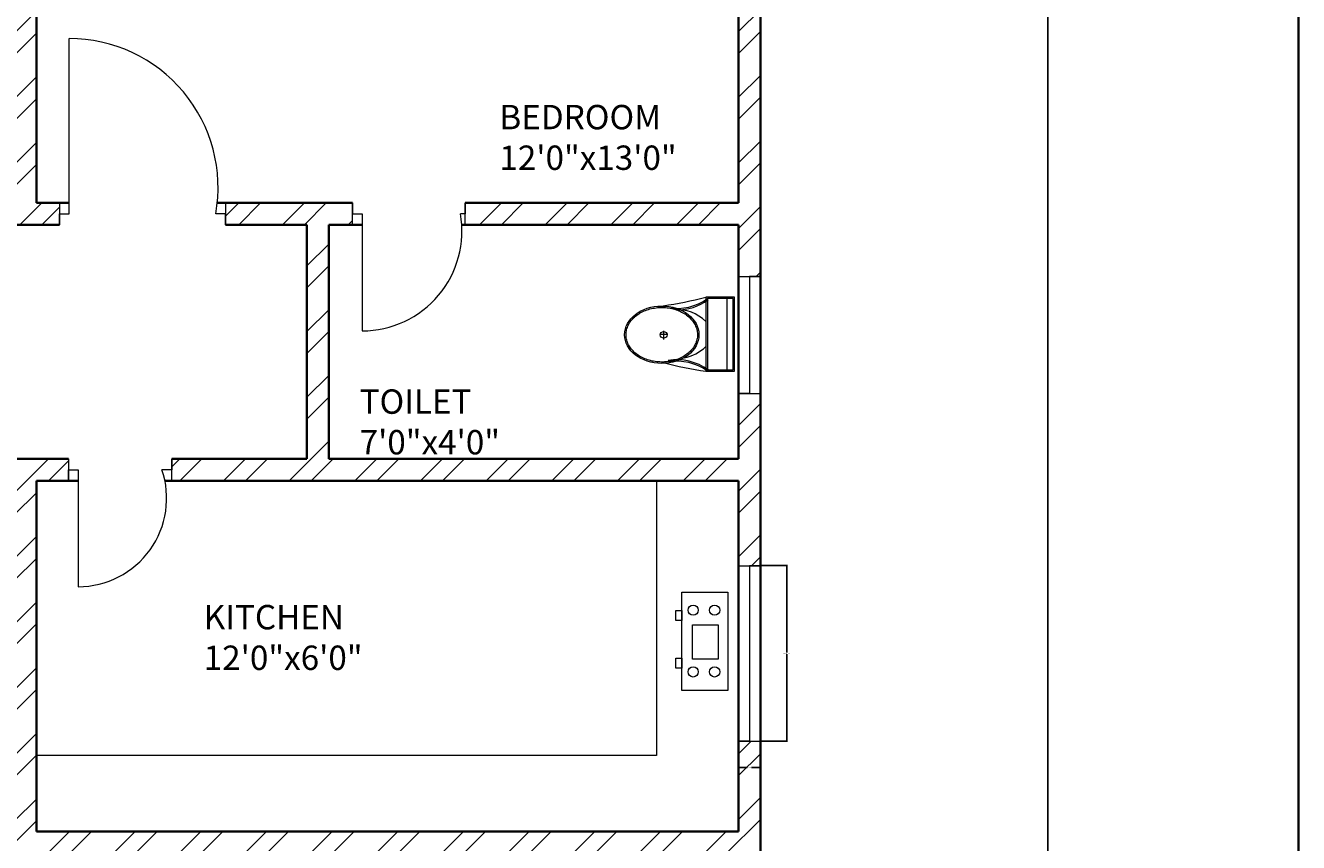
# Model space of a CAD drawing. Units: inches. Extents: x 1962 to 2771, y 1245 to 2660.
# Tile 112 of 114: x 2510 to 2771, y 2180 to 2348. Entities that reach past the tile are written whole.
import ezdxf

# ---------------------------------------------------------------- set-up
doc = ezdxf.new("R2010")
doc.units = ezdxf.units.IN
for name, color, linetype, lineweight in [('A-ANNO-DIMS', 2, 'Continuous', 18), ('A-ANNO-TTLB', 7, 'Continuous', 35), ('A-AREA-IDEN', 7, 'Continuous', 18), ('A-DOOR', 3, 'Continuous', 18), ('A-EQPM', 8, 'Continuous', 18), ('A-FLOR-CASE', 8, 'Continuous', 18), ('A-FLOR-FIXT', 8, 'Continuous', 18), ('A-GLAZ', 4, 'Continuous', 18), ('A-WALL', 7, 'Continuous', 35), ('A-WALL-PATT', 252, 'Continuous', 13)]:
    doc.layers.add(name, color=color, linetype=linetype, lineweight=lineweight)
doc.styles.get("Standard").update_dxf_attribs({"font": 'arial.ttf'})
doc.dimstyles.get("Standard").update_dxf_attribs({"dimtxt": 0.18, "dimasz": 0.18, "dimexe": 0.18, "dimexo": 0.0625, "dimgap": 0.09, "dimtad": 0, "dimtih": 1, "dimtoh": 1, "dimdec": 4, "dimzin": 0, "dimdsep": 46, "dimtxsty": 'Standard', "dimcen": 0.09, "dimadec": 0, "dimazin": 0, "dimtfac": 1, "dimtdec": 4, "dimtofl": 0, "dimtmove": 0, "dimatfit": 3, "dimfxl": 1, "dimtolj": 1, "dimtzin": 0, "dimarcsym": 0})

# ---------------------------------------------------------------- blocks, each defined once
blk = doc.blocks.new('A$C31115884')
for p, q in [((283.1, 497.7), (223.4, 497.7)), ((257.5, 466.4), (257.5, 523.2)), ((0, 200), (0, 0)), ((520, 200), (0, 200)), ((10, 190), (10, 10)), ((510, 190), (10, 190)), ((510, 10), (510, 190)), ((520, 0), (520, 200)), ((510, 54.5), (0, 54.5)), ((10, 10), (510, 10)), ((0, 0), (520, 0))]:
    blk.add_line(p, q)
blk.add_circle((255.6, 496.4), 23.6)
for centre, radius, start, end in [((2777.7, -204.6), 2807, 165.4549, 171.71327), ((-294.5, 403.3), 364.7, 324.20913, 9.34987), ((-294.5, 403.3), 374.7, 324.20913, 9.34987), ((805.8, 403.3), 364.7, 170.65013, 215.79087), ((3237, 905), 2807, 188.28673, 194.5451), ((139.5, 406.2), 293.5, 315.84364, 2.65635), ((805.8, 403.3), 374.7, 179.20365, 215.79087), ((383.6, 406.2), 293.5, 190.27735, 224.15636)]:
    blk.add_arc(centre, radius, start, end)
blk.add_ellipse((256.2, 509.9), major_axis=(0, -260.7), ratio=0.772727)
blk.add_open_spline([(256.2, 259.2), (263.1, 259.2), (270, 259.7), (287.8, 262.3), (298.7, 265.1), (319.9, 273.1), (330.2, 278.4), (350.1, 291.1), (359.7, 298.7), (377.7, 315.9), (386.2, 325.5), (401.7, 346.6), (408.8, 358.1), (421.3, 382.5), (426.8, 395.5), (435.9, 422.4), (439.5, 436.4), (444.8, 465.1), (446.5, 479.7), (447.9, 509.2), (447.6, 524), (445, 553.3), (442.7, 567.8), (436.3, 596), (432.1, 609.7), (421.9, 636), (416, 648.6), (402.5, 672.1), (395, 683), (378.6, 703), (369.8, 712.1), (351.1, 728), (341.3, 734.8), (320.9, 746.2), (310.4, 750.7), (288.9, 757.3), (278, 759.4), (256, 761), (245, 760.6), (223.1, 757.2), (212.3, 754.3), (191.1, 746.1), (180.8, 740.7), (160.9, 727.8), (151.4, 720.1), (133.5, 702.7), (125.1, 693), (109.6, 671.7), (102.6, 660.2), (90.2, 635.7), (84.9, 622.7), (76, 595.6), (72.4, 581.6), (67.2, 552.9), (65.6, 538.2), (64.4, 508.8), (64.8, 494), (67.5, 464.7), (69.9, 450.2), (76.6, 422), (80.8, 408.3), (91.1, 382.2), (97.2, 369.7), (110.8, 346.3), (118.4, 335.4), (134.8, 315.6), (143.7, 306.7), (162.4, 290.9), (172.3, 284.2), (192.8, 273), (203.3, 268.6), (224.8, 262.2), (235.8, 260.2), (249.9, 259.3), (253, 259.2), (256.2, 259.2)], degree=3, knots=[0, 0, 0, 0, 0.110105, 0.110105, 0.285049, 0.285049, 0.459994, 0.459994, 0.634938, 0.634938, 0.809882, 0.809882, 0.984827, 0.984827, 1.159771, 1.159771, 1.334715, 1.334715, 1.50966, 1.50966, 1.684604, 1.684604, 1.859549, 1.859549, 2.034493, 2.034493, 2.209437, 2.209437, 2.384382, 2.384382, 2.559326, 2.559326, 2.73427, 2.73427, 2.909215, 2.909215, 3.084159, 3.084159, 3.259103, 3.259103, 3.434048, 3.434048, 3.608992, 3.608992, 3.783936, 3.783936, 3.958881, 3.958881, 4.133825, 4.133825, 4.30877, 4.30877, 4.483714, 4.483714, 4.658658, 4.658658, 4.833603, 4.833603, 5.008547, 5.008547, 5.183491, 5.183491, 5.358436, 5.358436, 5.53338, 5.53338, 5.708324, 5.708324, 5.883269, 5.883269, 6.058213, 6.058213, 6.233158, 6.233158, 6.283185, 6.283185, 6.283185, 6.283185])
blk = doc.blocks.new('COOKTOP-4-BURNER')
for points in [[(0, 20.18), (9.48, 20.18), (9.48, 0), (0, 0)], [(2, 13.79), (7.26, 13.79), (7.26, 6.73), (2, 6.73)], [(9.48, 15.59), (10.71, 15.59), (10.71, 13.59), (9.48, 13.59)], [(9.48, 5.81), (10.71, 5.81), (10.71, 3.8), (9.48, 3.8)]]:
    blk.add_lwpolyline(points, close=True)
for centre in [(2.74, 16.38), (7.14, 16.38), (2.74, 3.71), (7.14, 3.71)]:
    blk.add_circle(centre, 1.05)
blk = doc.blocks.new('WIN-24IN-A')
for p, q in [((0, 24), (4.5, 24)), ((4.5, 24), (2.25, 24)), ((2.25, 24), (2.25, 0)), ((2.25, 0), (0, 0)), ((0, 0), (4.5, 0))]:
    blk.add_line(p, q)
blk = doc.blocks.new('WIN-36IN-B')
for p, q in [((0, 36), (4.5, 36)), ((4.5, 36), (2.25, 36)), ((2.25, 36), (2.25, 0)), ((2.25, 0), (0, 0)), ((0, 0), (4.5, 0))]:
    blk.add_line(p, q)
blk = doc.blocks.new('*D28')
at = {"layer": 'A-ANNO-DIMS', "color": 0, "lineweight": -2, "transparency": 16777216}
for p, q in [((2660.87, 2236.91), (2666.39, 2236.91)), ((2666.21, 2236.73), (2666.21, 2219.09)), ((2666.21, 2201.09), (2666.21, 2218.73)), ((2660.87, 2200.91), (2666.39, 2200.91))]:
    blk.add_line(p, q, dxfattribs=at)
at = {"layer": 'A-ANNO-DIMS', "color": 0, "transparency": 16777216}
for points in [[(2666.18, 2236.73), (2666.24, 2236.73), (2666.21, 2236.91)], [(2666.18, 2201.09), (2666.24, 2201.09), (2666.21, 2200.91)]]:
    blk.add_solid(points, dxfattribs=at)
at = {"layer": 'Defpoints', "color": 0, "transparency": 16777216}
for p in [(2660.81, 2236.91), (2666.21, 2236.91), (2660.81, 2200.91)]:
    blk.add_point(p, dxfattribs=at)
at = {"layer": 'A-ANNO-DIMS', "color": 0, "transparency": 16777216, "insert": (2666.21, 2218.91), "char_height": 0.18, "attachment_point": 5}
blk.add_mtext('\\A1;W2B 36 TYP.', dxfattribs=at)
blk = doc.blocks.new('*D29')
at = {"layer": 'A-ANNO-DIMS', "color": 0, "lineweight": -2, "transparency": 16777216}
for p, q in [((2656.31, 2200.85), (2656.31, 2195.33)), ((2660.81, 2200.85), (2660.81, 2195.33)), ((2656.49, 2195.51), (2658.1, 2195.51)), ((2660.63, 2195.51), (2659.02, 2195.51))]:
    blk.add_line(p, q, dxfattribs=at)
at = {"layer": 'A-ANNO-DIMS', "color": 0, "transparency": 16777216}
for points in [[(2656.49, 2195.54), (2656.49, 2195.48), (2656.31, 2195.51)], [(2660.63, 2195.54), (2660.63, 2195.48), (2660.81, 2195.51)]]:
    blk.add_solid(points, dxfattribs=at)
at = {"layer": 'Defpoints', "color": 0, "transparency": 16777216}
for p in [(2656.31, 2200.91), (2660.81, 2200.91), (2660.81, 2195.51)]:
    blk.add_point(p, dxfattribs=at)
at = {"layer": 'A-ANNO-DIMS', "color": 0, "transparency": 16777216, "insert": (2658.56, 2195.51), "char_height": 0.18, "attachment_point": 5}
blk.add_mtext('\\A1;5 TYP.', dxfattribs=at)
blk = doc.blocks.new('*D40')
at = {"layer": 'A-ANNO-DIMS', "color": 0, "lineweight": -2, "transparency": 16777216}
for p, q in [((2072.02, 2033.91), (2072.02, 2583.47)), ((2072.2, 2583.29), (2366.02, 2583.29)), ((2660.63, 2583.29), (2366.81, 2583.29)), ((2660.81, 2524.41), (2660.81, 2583.47))]:
    blk.add_line(p, q, dxfattribs=at)
at = {"layer": 'A-ANNO-DIMS', "color": 0, "transparency": 16777216}
for points in [[(2072.2, 2583.32), (2072.2, 2583.26), (2072.02, 2583.29)], [(2660.63, 2583.32), (2660.63, 2583.26), (2660.81, 2583.29)]]:
    blk.add_solid(points, dxfattribs=at)
at = {"layer": 'Defpoints', "color": 0, "transparency": 16777216}
for p in [(2660.81, 2583.29), (2660.81, 2524.34), (2072.02, 2033.84)]:
    blk.add_point(p, dxfattribs=at)
at = {"layer": 'A-ANNO-DIMS', "color": 0, "transparency": 16777216, "insert": (2366.41, 2583.29), "char_height": 0.18, "attachment_point": 5}
blk.add_mtext('\\A1;588.8', dxfattribs=at)
blk = doc.blocks.new('*D42')
at = {"layer": 'A-ANNO-DIMS', "color": 0, "lineweight": -2, "transparency": 16777216}
for p, q in [((2660.87, 2524.34), (2719.94, 2524.34)), ((2719.76, 2524.16), (2719.76, 1979.28)), ((2719.76, 1434.02), (2719.76, 1978.91)), ((2660.87, 1433.84), (2719.94, 1433.84))]:
    blk.add_line(p, q, dxfattribs=at)
at = {"layer": 'A-ANNO-DIMS', "color": 0, "transparency": 16777216}
for points in [[(2719.73, 2524.16), (2719.79, 2524.16), (2719.76, 2524.34)], [(2719.73, 1434.02), (2719.79, 1434.02), (2719.76, 1433.84)]]:
    blk.add_solid(points, dxfattribs=at)
at = {"layer": 'Defpoints', "color": 0, "transparency": 16777216}
for p in [(2660.81, 2524.34), (2719.76, 2524.34), (2660.81, 1433.84)]:
    blk.add_point(p, dxfattribs=at)
at = {"layer": 'A-ANNO-DIMS', "color": 0, "transparency": 16777216, "insert": (2719.76, 1979.09), "char_height": 0.18, "attachment_point": 5}
blk.add_mtext('\\A1;1090.5', dxfattribs=at)

msp = doc.modelspace()

# ---------------------------------------------------------------- hatches: boundary and pattern name
at = {"layer": 'A-WALL-PATT'}
h = msp.add_hatch(dxfattribs=at)
h.set_pattern_fill('ANSI32', color=256)
h.paths.add_polyline_path([(2090.8074, 2467.3437), (2141.6481, 2467.3437), (2141.6481, 2469.5937), (2141.6481, 2471.8437), (2086.3074, 2471.8437), (2086.3074, 2422.5333), (2090.8074, 2422.5333)])
h.paths.add_polyline_path([(2282.7664, 2471.8437), (2204.8982, 2471.8437), (2204.8982, 2467.3437), (2234.8074, 2467.3437), (2234.8074, 2311.3437), (2228.7492, 2311.3437), (2228.7492, 2306.8437), (2234.8074, 2306.8437), (2331.9227, 2306.8437), (2331.9227, 2309.0937), (2331.9227, 2311.3437), (2239.3074, 2311.3437), (2239.3074, 2467.3437), (2282.7664, 2467.3437), (2282.7664, 2469.5937)])
h.paths.add_polyline_path([(2471.4531, 2519.8437), (2552.011, 2519.8437), (2564.3996, 2519.8437), (2564.3996, 2511.1389), (2568.8996, 2511.1389), (2568.8996, 2524.3437), (2466.9531, 2524.3437), (2466.9531, 2471.8437), (2450.0749, 2471.8437), (2446.4672, 2471.8437), (2446.4672, 2467.3437), (2450.0749, 2467.3437), (2475.9988, 2467.3437), (2475.9988, 2469.5937), (2475.9988, 2471.8437), (2471.4531, 2471.8437)])
h.paths.add_polyline_path([(2575.2231, 2469.5937), (2575.2231, 2471.8437), (2568.8996, 2471.8437), (2568.8996, 2487.1389), (2564.3996, 2487.1389), (2564.3996, 2471.8437), (2556.511, 2471.8437), (2499.2904, 2471.8437), (2499.2904, 2467.3437), (2507.8074, 2467.3437), (2507.8074, 2311.3437), (2414.863, 2311.3437), (2414.863, 2306.8437), (2512.3074, 2306.8437), (2517.0114, 2306.8437), (2517.0114, 2309.0937), (2517.0114, 2311.3437), (2512.3074, 2311.3437), (2512.3074, 2467.3437), (2575.2231, 2467.3437)])
h.paths.add_polyline_path([(2660.8074, 2471.8437), (2600.9602, 2471.8437), (2600.9602, 2467.3437), (2656.3074, 2467.3437), (2656.3074, 2432.5704), (2660.8074, 2432.5704)])
h.paths.add_polyline_path([(2660.8074, 2372.5704), (2656.3074, 2372.5704), (2656.3074, 2311.3437), (2600.276, 2311.3437), (2600.276, 2309.0937), (2600.276, 2306.8437), (2656.3074, 2306.8437), (2656.3074, 2296.2593), (2660.8074, 2296.2593)])
h.paths.add_polyline_path([(2572.3074, 2306.8437), (2577.1385, 2306.8437), (2577.1385, 2311.3437), (2551.082, 2311.3437), (2551.082, 2306.8437), (2567.8074, 2306.8437), (2567.8074, 2258.8437), (2540.0574, 2258.8437), (2540.0574, 2256.5937), (2540.0574, 2254.3437), (2567.8074, 2254.3437), (2656.3074, 2254.3437), (2656.3074, 2236.9085), (2660.8074, 2236.9085), (2660.8074, 2272.2593), (2656.3074, 2272.2593), (2656.3074, 2258.8437), (2572.3074, 2258.8437)])
h.paths.add_polyline_path([(2512.3074, 2254.3437), (2518.8716, 2254.3437), (2518.8716, 2256.5937), (2518.8716, 2258.8437), (2507.8074, 2258.8437), (2507.8074, 2177.8437), (2567.8074, 2177.8437), (2567.8074, 2172.9628), (2572.3074, 2172.9628), (2572.3074, 2177.8437), (2656.3074, 2177.8437), (2656.3074, 2166.4846), (2660.8074, 2166.4846), (2660.8074, 2200.9085), (2656.3074, 2200.9085), (2656.3074, 2182.3437), (2512.3074, 2182.3437)])
h.paths.add_polyline_path([(2656.3074, 2129.8437), (2572.3074, 2129.8437), (2572.3074, 2150.3044), (2570.0574, 2150.3044), (2567.8074, 2150.3044), (2567.8074, 2129.8437), (2507.8074, 2129.8437), (2507.8074, 2116.3027), (2510.0574, 2116.3027), (2512.3074, 2116.3027), (2512.3074, 2125.3437), (2567.8074, 2125.3437), (2572.3074, 2125.3437), (2656.3074, 2125.3437)])
h.paths.add_polyline_path([(2090.8074, 2362.5333), (2086.3074, 2362.5333), (2086.3074, 2298.6242), (2090.8074, 2298.6242), (2090.8074, 2306.8437), (2174.8074, 2306.8437), (2174.8074, 2286.4178), (2179.3074, 2286.4178), (2179.3074, 2306.8437), (2192.8641, 2306.8437), (2192.8641, 2309.0937), (2192.8641, 2311.3437), (2090.8074, 2311.3437)])
h.paths.add_polyline_path([(2209.156, 2258.8437), (2179.3074, 2258.8437), (2179.3074, 2263.2236), (2177.0574, 2263.2236), (2174.8074, 2263.2236), (2174.8074, 2258.8437), (2090.8074, 2258.8437), (2090.8074, 2274.6242), (2086.3074, 2274.6242), (2086.3074, 2238.2967), (2088.5574, 2238.2967), (2090.8074, 2238.2967), (2090.8074, 2254.3437), (2209.156, 2254.3437)])
h.paths.add_polyline_path([(2090.8074, 2177.8437), (2234.8074, 2177.8437), (2234.8074, 2173.1428), (2239.3074, 2173.1428), (2239.3074, 2258.8437), (2230.8442, 2258.8437), (2230.8442, 2256.5937), (2230.8442, 2254.3437), (2234.8074, 2254.3437), (2234.8074, 2182.3437), (2090.8074, 2182.3437), (2090.8074, 2202.2967), (2086.3074, 2202.2967), (2086.3074, 2140.0389), (2090.8074, 2140.0389)])
h.paths.add_polyline_path([(2090.8074, 2080.0389), (2086.3074, 2080.0389), (2086.3074, 2033.8437), (2090.8074, 2033.8437)], flags=17)
h.paths.add_polyline_path([(2244.9405, 2033.8437), (2239.3074, 2033.8437), (2239.3074, 2142.0665), (2237.2592, 2142.0665), (2234.8074, 2142.0665), (2234.8074, 2033.8437), (2090.8074, 2033.8437), (2076.5204, 2033.8437), (2072.0204, 2033.8437), (2072.0204, 2000.4493), (2076.5204, 2000.4493), (2076.5204, 2029.3437), (2090.8074, 2029.3437), (2244.9405, 2029.3437), (2244.9405, 2031.5937)])
h.paths.add_polyline_path([(2234.8074, 1933.3437), (2076.5204, 1933.3437), (2076.5204, 1952.4493), (2074.2704, 1952.4493), (2072.0204, 1952.4493), (2072.0204, 1933.3437), (2072.0204, 1928.8437), (2234.8074, 1928.8437)])
h.paths.add_polyline_path([(2090.8074, 1928.8437), (2086.3074, 1928.8437), (2086.3074, 1906.5013), (2090.8074, 1906.5013)])
h.paths.add_polyline_path([(2090.8074, 1846.5013), (2086.3074, 1846.5013), (2086.3074, 1769.9917), (2088.5574, 1769.9917), (2090.8074, 1769.9917), (2090.8074, 1780.3437), (2234.8074, 1780.3437), (2234.8074, 1708.3437), (2230.3764, 1708.3437), (2230.3764, 1703.8437), (2239.3074, 1703.8437), (2239.3074, 1792.6669), (2237.0574, 1792.6669), (2234.8074, 1792.6669), (2234.8074, 1784.8437), (2090.8074, 1784.8437)])
h.paths.add_polyline_path([(2239.3074, 1928.8437), (2244.9405, 1928.8437), (2244.9405, 1931.0937), (2244.9405, 1933.3437), (2234.8074, 1933.3437), (2234.8074, 1928.8437), (2234.8074, 1825.5949), (2239.3074, 1825.5949)])
h.paths.add_polyline_path([(2148.0425, 1649.0937), (2148.0425, 1651.3437), (2090.8074, 1651.3437), (2090.8074, 1646.8437), (2148.0425, 1646.8437)], flags=0)
h.paths.add_polyline_path([(2207.5601, 1708.3437), (2090.8074, 1708.3437), (2090.8074, 1703.8437), (2174.8074, 1703.8437), (2174.8074, 1651.3437), (2170.4457, 1651.3437), (2170.4457, 1646.8437), (2195.9924, 1646.8437), (2195.9924, 1649.0937), (2195.9924, 1651.3437), (2179.3074, 1651.3437), (2179.3074, 1703.8437), (2207.5601, 1703.8437), (2207.5601, 1706.0937)])
h.paths.add_polyline_path([(2090.8074, 1733.9917), (2086.3074, 1733.9917), (2086.3074, 1696.1032), (2088.5574, 1696.1032), (2090.8074, 1696.1032)])
h.paths.add_polyline_path([(2090.8074, 1672.1032), (2086.3074, 1672.1032), (2086.3074, 1600.3335), (2090.8074, 1600.3335)])
h.paths.add_polyline_path([(2090.8074, 1540.3335), (2086.3074, 1540.3335), (2086.3074, 1486.3437), (2139.6766, 1486.3437), (2139.6766, 1490.8437), (2090.8074, 1490.8437)])
h.paths.add_polyline_path([(2302.3876, 1490.8437), (2239.3074, 1490.8437), (2239.3074, 1646.8437), (2335.9994, 1646.8437), (2335.9994, 1651.3437), (2229.884, 1651.3437), (2229.884, 1646.8437), (2234.8074, 1646.8437), (2234.8074, 1490.8437), (2202.7103, 1490.8437), (2202.7103, 1488.5937), (2202.7103, 1486.3437), (2275.0699, 1486.3437), (2275.0699, 1475.772), (2279.5699, 1475.772), (2279.5699, 1486.3437), (2302.3876, 1486.3437)])
h.paths.add_polyline_path([(2279.5699, 1451.772), (2275.0699, 1451.772), (2275.0699, 1438.3437), (2174.8074, 1438.3437), (2174.8074, 1486.3437), (2179.7922, 1486.3437), (2179.7922, 1490.8437), (2163.3585, 1490.8437), (2163.3585, 1488.5937), (2163.3585, 1486.3437), (2170.3074, 1486.3437), (2170.3074, 1433.8437), (2279.5699, 1433.8437)])
h.paths.add_polyline_path([(2427.2363, 1490.8437), (2375.8074, 1490.8437), (2375.8074, 1646.8437), (2381.6401, 1646.8437), (2381.6401, 1651.3437), (2365.887, 1651.3437), (2365.887, 1649.0937), (2365.887, 1646.8437), (2371.3074, 1646.8437), (2371.3074, 1490.8437), (2327.5627, 1490.8437), (2327.5627, 1488.5937), (2327.5627, 1486.3437), (2371.3074, 1486.3437), (2371.3074, 1433.8437), (2375.8074, 1433.8437), (2375.8074, 1486.3437), (2427.2363, 1486.3437)])
h.paths.add_polyline_path([(2512.3074, 1646.8437), (2519.4351, 1646.8437), (2519.4351, 1649.0937), (2519.4351, 1651.3437), (2507.8074, 1651.3437), (2416.0063, 1651.3437), (2416.0063, 1649.0937), (2416.0063, 1646.8437), (2507.8074, 1646.8437), (2507.8074, 1490.8437), (2497.0532, 1490.8437), (2497.0532, 1488.5937), (2497.0532, 1486.3437), (2574.9344, 1486.3437), (2574.9344, 1476.0181), (2579.4344, 1476.0181), (2579.4344, 1486.3437), (2584.4872, 1486.3437), (2584.3074, 1490.8437), (2512.3074, 1490.8437)])
h.paths.add_polyline_path([(2470.5091, 1486.3437), (2473.9767, 1486.3437), (2473.9767, 1490.8437), (2449.6605, 1490.8437), (2449.6605, 1488.5937), (2449.6605, 1486.3437), (2466.0091, 1486.3437), (2466.0091, 1433.8437), (2470.5091, 1433.8437), (2579.4344, 1433.8437), (2579.4344, 1452.0181), (2574.9344, 1452.0181), (2574.9344, 1438.3437), (2554.5091, 1438.3437), (2470.5091, 1438.3437)])
h.paths.add_polyline_path([(2656.3074, 1490.8437), (2611.86, 1490.8437), (2611.86, 1486.3437), (2656.3074, 1486.3437)])
h.paths.add_polyline_path([(2660.8074, 1532.7007), (2658.5574, 1532.7007), (2656.3074, 1532.7007), (2656.3074, 1486.3437), (2660.8074, 1486.3437)])
h.paths.add_polyline_path([(2660.8074, 1664.9663), (2656.3074, 1664.9663), (2656.3074, 1651.3437), (2602.2313, 1651.3437), (2602.2313, 1646.8437), (2656.3074, 1646.8437), (2656.3074, 1592.7007), (2660.8074, 1592.7007)])
h.paths.add_polyline_path([(2660.8074, 1724.5221), (2656.3074, 1724.5221), (2656.3074, 1703.8437), (2542.4725, 1703.8437), (2542.4725, 1699.3437), (2567.8074, 1699.3437), (2567.8074, 1651.3437), (2552.7766, 1651.3437), (2552.7766, 1649.0937), (2552.7766, 1646.8437), (2577.2878, 1646.8437), (2577.2878, 1649.0937), (2577.2878, 1651.3437), (2572.3074, 1651.3437), (2572.3074, 1699.3437), (2656.3074, 1699.3437), (2656.3074, 1688.9663), (2660.8074, 1688.9663)])
h.paths.add_polyline_path([(2660.8074, 1880.6524), (2656.3074, 1880.6524), (2656.3074, 1832.8437), (2512.3074, 1832.8437), (2512.3074, 1837.8959), (2507.8074, 1837.8959), (2507.8074, 1828.3437), (2567.8074, 1828.3437), (2567.8074, 1804.3437), (2572.3074, 1804.3437), (2572.3074, 1828.3437), (2656.3074, 1828.3437), (2656.3074, 1818.6778), (2660.8074, 1818.6778)])
h.paths.add_polyline_path([(2660.8074, 1794.6778), (2656.3074, 1794.6778), (2656.3074, 1780.3437), (2572.3074, 1780.3437), (2572.3074, 1783.0303), (2570.0574, 1783.0303), (2567.8074, 1783.0303), (2567.8074, 1780.3437), (2507.8074, 1780.3437), (2507.8074, 1699.3437), (2517.8858, 1699.3437), (2517.8858, 1701.5937), (2517.8858, 1703.8437), (2512.3074, 1703.8437), (2512.3074, 1775.8437), (2656.3074, 1775.8437), (2656.3074, 1760.5221), (2660.8074, 1760.5221)])
h.paths.add_polyline_path([(2660.8074, 1981.3437), (2660.8074, 2020.2808), (2658.5574, 2020.2808), (2656.3074, 2020.2808), (2656.3074, 1981.3437), (2512.3074, 1981.3437), (2512.3074, 2086.6996), (2507.8074, 2086.6996), (2507.8074, 1981.3437), (2375.8074, 1981.3437), (2375.8074, 1986.8505), (2373.5574, 1986.8505), (2371.3074, 1986.8505), (2371.3074, 1973.2607), (2375.8074, 1973.2607), (2375.8074, 1976.8437), (2507.8074, 1976.8437), (2507.8074, 1865.4281), (2510.0574, 1865.4281), (2512.3074, 1865.4281), (2512.3074, 1976.8437), (2660.8074, 1976.8437)])
h.paths.add_polyline_path([(2375.8074, 1940.297), (2373.5574, 1940.297), (2371.3074, 1940.297), (2371.3074, 1933.3437), (2278.4434, 1933.3437), (2278.4434, 1928.8437), (2371.3074, 1928.8437), (2371.3074, 1651.3437), (2375.8074, 1651.3437)])
h.paths.add_polyline_path([(2660.8074, 1976.8437), (2656.3074, 1976.8437), (2656.3074, 1940.6524), (2660.8074, 1940.6524)], flags=17)
h.paths.add_polyline_path([(2660.8074, 2142.4846), (2656.3074, 2142.4846), (2656.3074, 2080.2808), (2660.8074, 2080.2808)])
h.paths.add_polyline_path([(2381.4189, 2311.3437), (2375.8074, 2311.3437), (2375.8074, 2467.3437), (2424.7242, 2467.3437), (2424.7242, 2469.5937), (2424.7242, 2471.8437), (2375.8074, 2471.8437), (2375.8074, 2524.3437), (2371.3074, 2524.3437), (2371.3074, 2471.8437), (2307.2097, 2471.8437), (2307.2097, 2467.3437), (2371.3074, 2467.3437), (2371.3074, 2311.3437), (2366.8901, 2311.3437), (2366.8901, 2306.8437), (2371.3074, 2306.8437), (2371.3074, 2033.8437), (2279.6589, 2033.8437), (2279.6589, 2029.3437), (2371.3074, 2029.3437), (2371.3074, 2014.2598), (2375.8074, 2014.2598), (2375.8074, 2306.8437), (2381.4189, 2306.8437)])
h.paths.add_polyline_path([(2263.3074, 2524.3437), (2170.3074, 2524.3437), (2170.3074, 2519.8437), (2170.3074, 2471.8437), (2165.0312, 2471.8437), (2165.0312, 2467.3437), (2179.6721, 2467.3437), (2179.6721, 2469.5161), (2179.6721, 2471.8437), (2174.8074, 2471.8437), (2174.8074, 2519.8437), (2258.8074, 2519.8437), (2258.8074, 2511.6436), (2263.3074, 2511.6436)])
h.paths.add_polyline_path([(2245.0232, 1361.4123), (2492.9468, 1361.4123), (2492.9468, 1398.505), (2245.0232, 1398.505)], flags=9)
h.paths.add_polyline_path([(2388.1434, 2086.6936), (2425.0704, 2086.6936), (2425.0704, 2105.3509), (2388.1434, 2105.3509)], flags=9)
h.paths.add_polyline_path([(2404.922, 2242.6744), (2445.7337, 2242.6744), (2445.7337, 2261.3318), (2404.922, 2261.3318)], flags=9)
h.paths.add_polyline_path([(2269.4107, 2156.7935), (2306.3378, 2156.7935), (2306.3378, 2175.4508), (2269.4107, 2175.4508)], flags=9)
h.paths.add_polyline_path([(2269.3277, 2233.4343), (2306.2547, 2233.4343), (2306.2547, 2252.0917), (2269.3277, 2252.0917)], flags=9)
h.paths.add_polyline_path([(2431.6052, 2320.6922), (2470.4456, 2320.6922), (2470.4456, 2339.3495), (2431.6052, 2339.3495)], flags=25)
h.paths.add_polyline_path([(2249.6902, 2315.7608), (2288.5306, 2315.7608), (2288.5306, 2334.4182), (2249.6902, 2334.4182)], flags=25)
h.paths.add_polyline_path([(2096.9301, 2314.3181), (2135.7704, 2314.3181), (2135.7704, 2332.9755), (2096.9301, 2332.9755)], flags=25)
h.paths.add_polyline_path([(2134.3475, 2285.7089), (2161.4655, 2285.7089), (2161.4655, 2304.3662), (2134.3475, 2304.3662)], flags=9)
h.paths.add_polyline_path([(2126.5155, 2209.4076), (2159.9227, 2209.4076), (2159.9227, 2228.065), (2126.5155, 2228.065)], flags=25)
h.paths.add_polyline_path([(2110.5753, 2141.5299), (2149.4157, 2141.5299), (2149.4157, 2160.1872), (2110.5753, 2160.1872)], flags=25)
h.paths.add_polyline_path([(2249.8618, 1968.3317), (2286.3966, 1968.3317), (2286.3966, 1986.989), (2249.8618, 1986.989)], flags=9)
h.paths.add_polyline_path([(2395.9507, 1777.0051), (2436.7624, 1777.0051), (2436.7624, 1795.6625), (2395.9507, 1795.6625)], flags=9)
h.paths.add_polyline_path([(2398.5259, 1888.5651), (2435.0062, 1888.5651), (2435.0062, 1907.2224), (2398.5259, 1907.2224)], flags=25)
h.paths.add_polyline_path([(2259.3506, 1728.3559), (2296.2776, 1728.3559), (2296.2776, 1747.0132), (2259.3506, 1747.0132)], flags=9)
h.paths.add_polyline_path([(2271.3698, 1845.268), (2308.2968, 1845.268), (2308.2968, 1863.9253), (2271.3698, 1863.9253)], flags=9)
h.paths.add_polyline_path([(2120.9355, 1786.3027), (2159.7759, 1786.3027), (2159.7759, 1804.9601), (2120.9355, 1804.9601)], flags=25)
h.paths.add_polyline_path([(2121.3164, 1732.1043), (2154.7236, 1732.1043), (2154.7236, 1750.7616), (2121.3164, 1750.7616)], flags=25)
h.paths.add_polyline_path([(2118.3706, 1678.8997), (2147.5282, 1678.8997), (2147.5282, 1697.557), (2118.3706, 1697.557)], flags=25)
h.paths.add_polyline_path([(2385.9227, 1493.557), (2424.763, 1493.557), (2424.763, 1512.2143), (2385.9227, 1512.2143)], flags=25)
h.paths.add_polyline_path([(2248.7058, 1500.0256), (2287.5462, 1500.0256), (2287.5462, 1518.6829), (2248.7058, 1518.6829)], flags=25)
h.paths.add_polyline_path([(2104.1669, 1617.3771), (2143.0073, 1617.3771), (2143.0073, 1636.0344), (2104.1669, 1636.0344)], flags=9)
h.paths.add_polyline_path([(2096.0714, 1447.8824), (2137.3845, 1447.8824), (2137.3845, 1458.1859), (2096.0714, 1458.1859)], flags=9)
h.paths.add_polyline_path([(2180.6114, 1440.325), (2209.7689, 1440.325), (2209.7689, 1458.9823), (2180.6114, 1458.9823)], flags=25)
h.paths.add_polyline_path([(2316.1698, 1447.9637), (2357.4829, 1447.9637), (2357.4829, 1458.2673), (2316.1698, 1458.2673)], flags=9)
h.paths.add_polyline_path([(2397.6187, 1447.9637), (2438.9318, 1447.9637), (2438.9318, 1458.2673), (2397.6187, 1458.2673)], flags=9)
h.paths.add_polyline_path([(2473.0778, 1439.5953), (2502.2354, 1439.5953), (2502.2354, 1458.2527), (2473.0778, 1458.2527)], flags=25)
h.paths.add_polyline_path([(2589.7027, 1447.8819), (2631.0158, 1447.8819), (2631.0158, 1458.1855), (2589.7027, 1458.1855)], flags=9)
h.paths.add_polyline_path([(2522.4009, 1497.5285), (2561.2413, 1497.5285), (2561.2413, 1516.1859), (2522.4009, 1516.1859)], flags=25)
h.paths.add_polyline_path([(2579.6565, 1671.3482), (2608.8141, 1671.3482), (2608.8141, 1690.0056), (2579.6565, 1690.0056)], flags=25)
h.paths.add_polyline_path([(2544.7038, 1725.5064), (2578.1111, 1725.5064), (2578.1111, 1744.1637), (2544.7038, 1744.1637)], flags=25)
h.paths.add_polyline_path([(2578.1191, 1807.472), (2607.2766, 1807.472), (2607.2766, 1826.1293), (2578.1191, 1826.1293)], flags=25)
h.paths.add_polyline_path([(2595.0614, 1835.1839), (2633.9018, 1835.1839), (2633.9018, 1853.8413), (2595.0614, 1853.8413)], flags=25)
h.paths.add_polyline_path([(2567.0097, 2097.7035), (2605.8501, 2097.7035), (2605.8501, 2116.3609), (2567.0097, 2116.3609)], flags=9)
h.paths.add_polyline_path([(2586.644, 2134.6454), (2615.8015, 2134.6454), (2615.8015, 2153.3027), (2586.644, 2153.3027)], flags=9)
h.paths.add_polyline_path([(2544.6185, 2212.6783), (2578.0258, 2212.6783), (2578.0258, 2231.3356), (2544.6185, 2231.3356)], flags=25)
h.paths.add_polyline_path([(2577.0273, 2256.9023), (2606.1849, 2256.9023), (2606.1849, 2275.5597), (2577.0273, 2275.5597)], flags=24)
h.paths.add_polyline_path([(2605.2683, 2315.2821), (2644.1087, 2315.2821), (2644.1087, 2333.9395), (2605.2683, 2333.9395)], flags=25)
h.paths.add_polyline_path([(2583.1244, 2496.1815), (2624.4375, 2496.1815), (2624.4375, 2506.4851), (2583.1244, 2506.4851)], flags=9)
h.paths.add_polyline_path([(2474.761, 2497.0823), (2503.9185, 2497.0823), (2503.9185, 2515.7397), (2474.761, 2515.7397)], flags=25)
h.paths.add_polyline_path([(2387.5787, 2494.2563), (2428.902, 2494.2563), (2428.902, 2504.5598), (2387.5787, 2504.5598)], flags=9)
h.paths.add_polyline_path([(2300.1657, 2500.1564), (2341.4788, 2500.1564), (2341.4788, 2510.46), (2300.1657, 2510.46)], flags=25)
h.paths.add_polyline_path([(2176.8589, 2497.5843), (2206.0165, 2497.5843), (2206.0165, 2516.2416), (2176.8589, 2516.2416)], flags=25)
h.paths.add_polyline_path([(2097.4668, 2494.9762), (2138.7799, 2494.9762), (2138.7799, 2505.2798), (2097.4668, 2505.2798)], flags=9)

# ---------------------------------------------------------------- linework, layer by layer
at = {"layer": 'A-ANNO-TTLB'}
msp.add_lwpolyline([(1961.7365, 2660.2579), (2771.213, 2660.2579), (2771.213, 1244.5817), (1961.7365, 1244.5817)], close=True, dxfattribs=at)
at = {"layer": 'A-DOOR'}
for p, q in [((2519.0114, 2309.0937), (2519.0114, 2345.0937)), ((2517.0114, 2311.3437), (2517.0114, 2306.8437)), ((2551.082, 2311.3437), (2551.082, 2306.8437)), ((2577.1385, 2306.8437), (2577.1385, 2311.3437)), ((2577.1385, 2311.3437), (2577.1385, 2309.0937)), ((2600.276, 2306.8437), (2600.276, 2311.3437)), ((2600.276, 2311.3437), (2600.276, 2309.0937)), ((2517.0114, 2306.8437), (2517.0114, 2309.0937)), ((2517.0114, 2309.0937), (2519.0114, 2309.0937)), ((2551.082, 2309.0937), (2549.082, 2309.0937)), ((2551.082, 2306.8437), (2551.082, 2309.0937)), ((2577.1385, 2309.0937), (2579.1385, 2309.0937)), ((2579.1385, 2309.0937), (2579.1385, 2285.0937)), ((2600.276, 2309.0937), (2599.276, 2309.0937)), ((2518.8716, 2258.8437), (2518.8716, 2254.3437)), ((2518.8716, 2254.3437), (2518.8716, 2256.5937)), ((2518.8716, 2256.5937), (2520.8716, 2256.5937)), ((2520.8716, 2256.5937), (2520.8716, 2232.5937)), ((2540.0574, 2256.5937), (2538.0574, 2256.5937)), ((2540.0574, 2254.3437), (2540.0574, 2258.8437)), ((2540.0574, 2258.8437), (2540.0574, 2256.5937))]:
    msp.add_line(p, q, dxfattribs=at)
for centre, radius, start, end in [((2519.0114, 2314.5348), 30.5589, 349.743657, 90), ((2579.1385, 2305.5421), 20.4484, 270, 10.002342), ((2520.8716, 2250.7468), 18.1531, 270, 18.789109)]:
    msp.add_arc(centre, radius, start, end, dxfattribs=at)
at = {"layer": 'A-FLOR-CASE'}
for p, q in [((2639.5039, 2254.3437), (2639.5039, 2197.9864)), ((2639.5039, 2197.9864), (2512.3074, 2197.9864))]:
    msp.add_line(p, q, dxfattribs=at)
at = {"layer": 'A-WALL'}
for p, q in [((2660.8074, 2471.8437), (2660.8074, 1976.8437)), ((2512.3074, 2467.3437), (2512.3074, 2311.3437)), ((2656.3074, 2467.3437), (2656.3074, 2311.3437)), ((2512.3074, 2311.3437), (2519.0114, 2311.3437)), ((2549.4032, 2311.3437), (2577.1385, 2311.3437)), ((2600.276, 2311.3437), (2656.3074, 2311.3437)), ((2414.863, 2306.8437), (2512.3074, 2306.8437)), ((2512.3074, 2306.8437), (2517.0114, 2306.8437)), ((2551.082, 2306.8437), (2567.8074, 2306.8437)), ((2567.8074, 2306.8437), (2567.8074, 2258.8437)), ((2572.3074, 2258.8437), (2572.3074, 2306.8437)), ((2572.3074, 2306.8437), (2579.1385, 2306.8437)), ((2599.5454, 2306.8437), (2656.3074, 2306.8437)), ((2656.3074, 2306.8437), (2656.3074, 2258.8437)), ((2518.8716, 2258.8437), (2507.8074, 2258.8437)), ((2567.8074, 2258.8437), (2540.0574, 2258.8437)), ((2572.3074, 2258.8437), (2656.3074, 2258.8437)), ((2512.3074, 2254.3437), (2512.3074, 2182.3437)), ((2520.8716, 2254.3437), (2512.3074, 2254.3437)), ((2567.8074, 2254.3437), (2538.6648, 2254.3437)), ((2567.8074, 2254.3437), (2656.3074, 2254.3437)), ((2656.3074, 2254.3437), (2656.3074, 2182.3437)), ((2512.3074, 2182.3437), (2656.3074, 2182.3437))]:
    msp.add_line(p, q, dxfattribs=at)

# ---------------------------------------------------------------- block references
at = {"layer": 'A-EQPM', "rotation": 180}
msp.add_blockref('COOKTOP-4-BURNER', (2654.1701, 2231.4915), dxfattribs=at)
at = {"layer": 'A-FLOR-FIXT', "xscale": 0.0292470664339069, "yscale": 0.0292470664339069, "zscale": 0.0292470664339069, "rotation": 89.99999999999999}
msp.add_blockref('A$C31115884', (2655.4994, 2276.8006), dxfattribs=at)
at = {"layer": 'A-GLAZ'}
for name, p in [('WIN-24IN-A', (2656.3074, 2272.2593)), ('WIN-36IN-B', (2656.3074, 2200.9085))]:
    msp.add_blockref(name, p, dxfattribs=at)

# ---------------------------------------------------------------- texts
at = {"layer": 'A-AREA-IDEN', "char_height": 5, "attachment_point": 1}
for s, width, insert in [('BEDROOM\\P12\'0"x13\'0"', 115.390761, (2607.2789, 2331.4548)), ('TOILET\\P7\'0"x4\'0"', 138.595395, (2578.6082, 2273.075)), ('KITCHEN\\P12\'0"x6\'0"', 148.093554, (2546.6291, 2228.8475))]:
    msp.add_mtext_dynamic_manual_height_columns(s, width=width, gutter_width=12.5, heights=[0], dxfattribs=dict(at, insert=insert))

# ---------------------------------------------------------------- dimensions: what is measured, and where the dimension line sits
at = {"layer": 'A-ANNO-DIMS'}
dim = msp.add_linear_dim(base=(2660.8074, 2583.2937), p1=(2072.0204, 2033.8437), p2=(2660.8074, 2524.3437), dimstyle='Standard', override={"dimdec": 1, "dimlfac": 1, "dimrnd": 0, "dimzin": 0, "dimdsep": 46, "dimlunit": 2}, dxfattribs=at)
dim.commit()
dim.dimension.update_dxf_attribs({"geometry": '*D40', "text_midpoint": (2366.4139, 2583.2937)})
dim = msp.add_linear_dim(base=(2719.7574, 2524.3437), p1=(2660.8074, 1433.8437), p2=(2660.8074, 2524.3437), angle=90, dimstyle='Standard', override={"dimdec": 1, "dimlfac": 1, "dimrnd": 0, "dimzin": 0, "dimdsep": 46, "dimlunit": 2}, dxfattribs=at)
dim.commit()
dim.dimension.update_dxf_attribs({"geometry": '*D42', "text_midpoint": (2719.7574, 1979.0937)})
dim = msp.add_linear_dim(base=(2666.2074, 2236.9085), p1=(2660.8074, 2200.9085), p2=(2660.8074, 2236.9085), angle=90, text='W2B <> TYP.', dimstyle='Standard', override={"dimdec": 0, "dimlfac": 1, "dimrnd": 0, "dimzin": 0, "dimdsep": 46, "dimlunit": 2}, dxfattribs=at)
dim.commit()
dim.dimension.update_dxf_attribs({"geometry": '*D28', "text_midpoint": (2666.2074, 2218.9085)})
dim = msp.add_linear_dim(base=(2660.8073805882, 2195.5084878949), p1=(2656.3073805882, 2200.9084878949), p2=(2660.8073805882, 2200.9084878949), text='<> TYP.', dimstyle='Standard', override={"dimdec": 0, "dimlfac": 1, "dimrnd": 0, "dimzin": 0, "dimdsep": 46, "dimlunit": 2}, dxfattribs=at)
dim.commit()
dim.dimension.update_dxf_attribs({"geometry": '*D29', "text_midpoint": (2658.5573805882, 2195.5084878949)})

doc.saveas('drawing.dxf')
